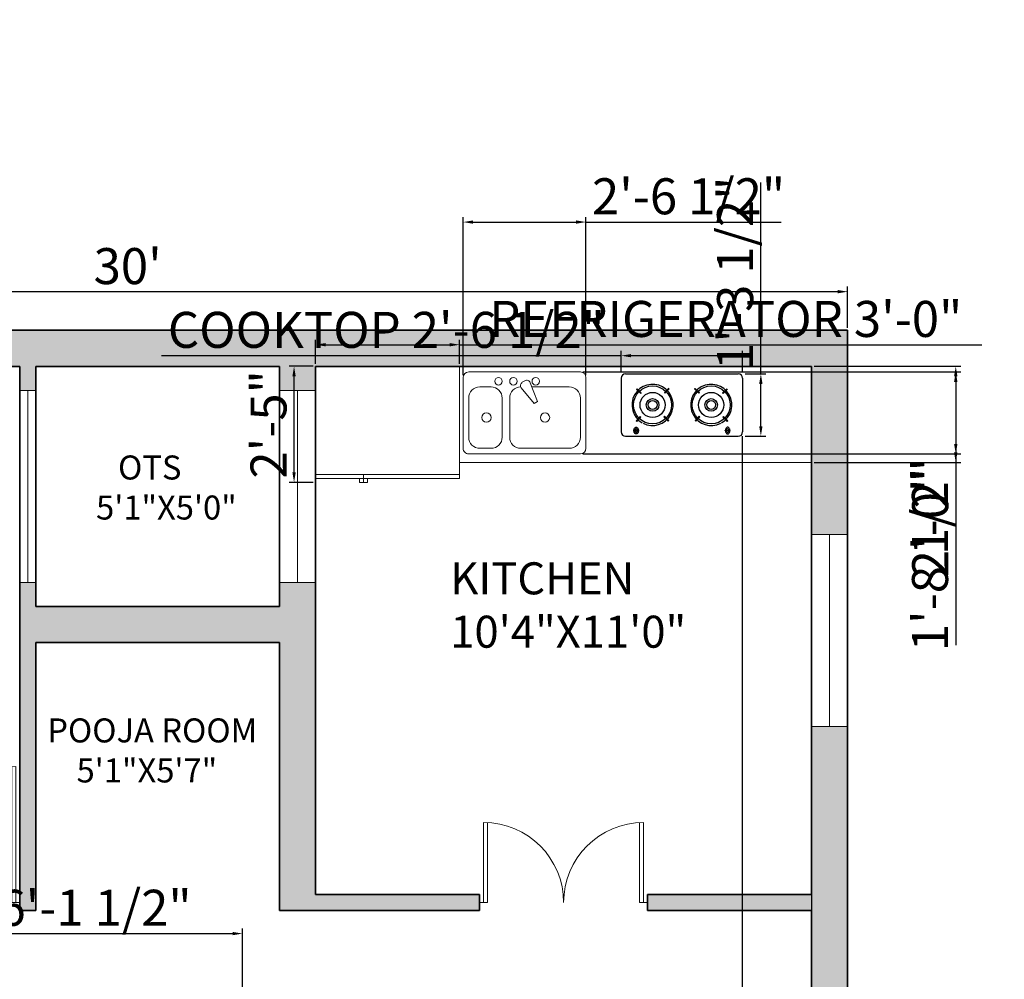
# Model space of a CAD drawing. Units: inches. Extents: x 3592 to 4861, y 1650 to 2243.
# Tile 25 of 30: x 4191 to 4438, y 2003 to 2243. Entities that reach past the tile are written whole.
import ezdxf

# ---------------------------------------------------------------- set-up
doc = ezdxf.new("R2010")
doc.units = ezdxf.units.IN
for name, color, linetype, lineweight in [('A-ANNO-DIMS', 2, 'Continuous', 13), ('A-AREA-IDEN', 7, 'Continuous', 18), ('A-DOOR', 3, 'Continuous', 20), ('A-FLOR-CASE', 7, 'Continuous', 18), ('A-GLAZ', 4, 'Continuous', 18), ('A-WALL', 7, 'Continuous', 35), ('THIET-BI', 21, 'Continuous', 18), ('Сантехника', 9, 'Continuous', 18)]:
    doc.layers.add(name, color=color, linetype=linetype, lineweight=lineweight)
doc.layers.add('A-WALL-PATT', color=252, linetype='Continuous', lineweight=13, true_color=0x939598)
doc.layers.add('NOI THAT', color=42, linetype='Continuous')
doc.styles.add('ATT', font='romans.shx')
doc.styles.get("Standard").update_dxf_attribs({"font": 'arial.ttf'})
doc.dimstyles.new('ISO-25', dxfattribs={"dimtxt": 9, "dimasz": 2.5, "dimexe": 1.25, "dimexo": 0.625, "dimtad": 1, "dimlunit": 3, "dimtxsty": 'Standard', "dimcen": 2.5, "dimadec": 0, "dimazin": 0, "dimtfac": 1, "dimtmove": 0, "dimatfit": 3, "dimfxl": 1, "dimarcsym": 0})

# ---------------------------------------------------------------- blocks, each defined once
blk = doc.blocks.new('1')
for p, q in [((3628.27, 1890.86), (3628.27, 1924.86)), ((3629.27, 1890.86), (3629.27, 1924.86)), ((3627.27, 1890.86), (3629.27, 1890.86)), ((3662.27, 1890.86), (3663.27, 1890.86))]:
    blk.add_line(p, q)
blk.add_arc((3628.27, 1890.86), 34, 0, 90)
blk = doc.blocks.new('MD')
for p, q in [((3665.34, 1831.69), (3665.34, 1851.69)), ((3666.34, 1831.69), (3666.34, 1851.69)), ((3704.34, 1831.69), (3704.34, 1851.69)), ((3705.34, 1831.69), (3705.34, 1851.69)), ((3664.34, 1831.69), (3666.34, 1831.69)), ((3706.34, 1831.69), (3704.34, 1831.69))]:
    blk.add_line(p, q)
for centre, start, end in [((3665.34, 1831.69), 0, 90), ((3705.34, 1831.69), 90, 180)]:
    blk.add_arc(centre, 20, start, end)
blk = doc.blocks.new('*D7')
at = {"layer": 'A-ANNO-DIMS', "color": 0, "lineweight": -2, "transparency": 16777216}
for p, q in [((4038.37, 2165.84), (4038.37, 2176.13)), ((4040.87, 2174.88), (4395.87, 2174.88)), ((4398.37, 2165.84), (4398.37, 2176.13))]:
    blk.add_line(p, q, dxfattribs=at)
at = {"layer": 'A-ANNO-DIMS', "color": 0, "transparency": 16777216}
for points in [[(4040.87, 2175.3), (4040.87, 2174.46), (4038.37, 2174.88)], [(4395.87, 2175.3), (4395.87, 2174.46), (4398.37, 2174.88)]]:
    blk.add_solid(points, dxfattribs=at)
at = {"layer": 'Defpoints', "color": 0, "transparency": 16777216}
for p in [(4398.37, 2174.88), (4038.37, 2165.22), (4398.37, 2165.22)]:
    blk.add_point(p, dxfattribs=at)
at = {"layer": 'A-ANNO-DIMS', "color": 0, "transparency": 16777216, "insert": (4218.37, 2180.1), "char_height": 9, "attachment_point": 5}
blk.add_mtext("30'", dxfattribs=at)
blk = doc.blocks.new('15PSNK11')
at = {"color": 0, "linetype": 'ByBlock'}
for p, q in [((1.5, 16.5), (20.5, 16.5)), ((0, -15), (0, 15)), ((17.5, 15), (7, 15)), ((22, 15), (22, -15)), ((4, 12), (4, 1.954648)), ((20.5, -1), (20.5, 12)), ((2.880753, 1.53534), (7.946152, 3.433013)), ((7.946152, 3.433013), (8.446152, 2.566987)), ((2.365551, 0.098898), (2.768424, -0.598898)), ((8.446152, 2.566987), (4.27002, -0.870941)), ((7, -4), (17.5, -4)), ((17.5, -6), (7, -6)), ((4, -9), (4, -12)), ((20.5, -12), (20.5, -9)), ((7, -15), (17.5, -15)), ((20.5, -16.5), (1.5, -16.5))]:
    blk.add_line(p, q, dxfattribs=at)
for centre, radius in [((12.25, 5.5), 1.25), ((2.5, 3), 1), ((2.5, -3), 1), ((2.5, -7), 1), ((12.25, -10.25), 1.25)]:
    blk.add_circle(centre, radius, dxfattribs=at)
for centre, radius, start, end in [((1.5, 15), 1.5, 90, 180), ((20.5, 15), 1.5, 0, 90), ((7, 12), 3, 90, 180), ((17.5, 12), 3, 0, 90), ((3.231576, 0.598898), 1, 110.537678, 210), ((3.634449, -0.098898), 1, 210, 309.462322), ((7, -1), 3, 180, 270), ((17.5, -1), 3, 270, 0), ((7, -9), 3, 90, 180), ((17.5, -9), 3, 0, 90), ((7, -12), 3, 180, 270), ((17.5, -12), 3, 270, 0), ((1.5, -15), 1.5, 180, 270), ((20.5, -15), 1.5, 270, 0)]:
    blk.add_arc(centre, radius, start, end, dxfattribs=at)
at = {"color": 0, "linetype": 'ByBlock', "style": 'ATT'}
for tag, p, flags in [('ITEM', (0, -26), 3), ('ROOM_NUMBER', (0, -35), 1)]:
    blk.add_attdef(tag, p, '', height=6, dxfattribs=dict(at, flags=flags))
blk = doc.blocks.new('A$C2C6C0730')
at = {"layer": 'NOI THAT'}
for p, q in [((670, 1403), (50, 1403)), ((0, 1353), (0, 50)), ((720, 1353), (720, 50)), ((670, 0), (50, 0))]:
    blk.add_line(p, q, dxfattribs=at)
for points in [[(66, 1257, -0.070182), (81, 1254, -0.081942), (93, 1249, -0.106897), (102, 1239, -0.135195), (105, 1230, -0.135195), (102, 1220, -0.106897), (93, 1210, -0.081942), (81, 1205, -0.070182), (66, 1203, -0.070182), (50, 1205, -0.081942), (38, 1210, -0.106897), (30, 1220, -0.135195), (27, 1230, -0.135195), (30, 1239, -0.106897), (38, 1249, -0.081942), (50, 1254, -0.070182)], [(66, 146, 0.070182), (81, 148, 0.081942), (93, 154, 0.106897), (102, 163, 0.135195), (105, 173, 0.135195), (102, 183, 0.106897), (93, 192, 0.081942), (81, 198, 0.070182), (66, 200, 0.070182), (50, 198, 0.081942), (38, 192, 0.106897), (30, 183, 0.135195), (27, 173, 0.135195), (30, 163, 0.106897), (38, 154, 0.081942), (50, 148, 0.070182)]]:
    blk.add_lwpolyline(points, format="xyb", close=True, dxfattribs=at)
for points in [[(68, 1203), (68, 1257), (62, 1257), (62, 1203)], [(220, 1175), (171, 1223), (179, 1230), (227, 1182)], [(541, 1226), (493, 1177), (500, 1170), (548, 1219)], [(176, 861), (224, 909), (232, 902), (183, 853)], [(497, 897), (546, 849), (553, 856), (505, 904)], [(176, 542), (224, 494), (232, 501), (183, 550)], [(497, 506), (546, 554), (553, 547), (505, 498)], [(220, 228), (171, 180), (179, 172), (227, 221)], [(541, 177), (493, 225), (500, 233), (548, 184)], [(68, 200), (68, 146), (62, 146), (62, 200)]]:
    blk.add_lwpolyline(points, close=True, dxfattribs=at)
for centre, radius in [((362, 1040), 219), ((362, 1040), 145), ((362, 1040), 72.6), ((362, 1040), 51.5), ((362, 363), 219), ((362, 363), 145), ((362, 363), 72.6), ((362, 363), 51.5)]:
    blk.add_circle(centre, radius, dxfattribs=at)
for centre, radius, start, end in [((50, 1353), 50, 90, 180), ((670, 1353), 50, 0, 90), ((362, 1040), 238, 152.4796, 149.9329), ((65, 1230), 19.4, 99.7177, 260.2823), ((65, 1230), 19.4, 279.9102, 80.0898), ((362, 363), 238, 210.0671, 207.5204), ((65, 173), 19.4, 99.7177, 260.2823), ((65, 173), 19.4, 279.9102, 80.0898), ((50, 50), 50, 180, 270), ((670, 50), 50, 270, 0)]:
    blk.add_arc(centre, radius, start, end, dxfattribs=at)
blk = doc.blocks.new('Refrigerator-2 door - 36 in top')
for p, q in [((0, -26.999999), (36, -26.999999)), ((12, -26.999999), (12, -28.999999)), ((11, -27.999999), (11, -28.999999)), ((11, -28.999999), (13, -28.999999)), ((13, -28.999999), (13, -27.999999))]:
    blk.add_line(p, q)
blk.add_lwpolyline([(0, -27.999999), (0, 0), (36, 0), (36, -27.999999)], close=True)
blk = doc.blocks.new('*D155')
at = {"layer": 'A-ANNO-DIMS', "color": 0, "lineweight": -2, "transparency": 16777216}
for p, q in [((4183.77, 2156.22), (4183.77, 2242.84)), ((4169.25, 2156.22), (4185.02, 2156.22)), ((4183.77, 2075.11), (4183.77, 2153.72)), ((4169.25, 2072.61), (4185.02, 2072.61))]:
    blk.add_line(p, q, dxfattribs=at)
at = {"layer": 'A-ANNO-DIMS', "color": 0, "transparency": 16777216}
for points in [[(4183.36, 2153.72), (4184.19, 2153.72), (4183.77, 2156.22)], [(4183.36, 2075.11), (4184.19, 2075.11), (4183.77, 2072.61)]]:
    blk.add_solid(points, dxfattribs=at)
at = {"layer": 'Defpoints', "color": 0, "transparency": 16777216}
for p in [(4168.62, 2156.22), (4183.77, 2156.22), (4168.62, 2072.61)]:
    blk.add_point(p, dxfattribs=at)
at = {"layer": 'A-ANNO-DIMS', "color": 0, "transparency": 16777216, "insert": (4178.5, 2200.78), "char_height": 9, "attachment_point": 5, "rotation": 90}
blk.add_mtext('6\'-11 1/2" TYP.', dxfattribs=at)
blk = doc.blocks.new('*D160')
at = {"layer": 'A-ANNO-DIMS', "color": 0, "lineweight": -2, "transparency": 16777216}
for p, q in [((4341.76, 2154.95), (4341.76, 2160.13)), ((4372.13, 2154.95), (4372.13, 2160.13)), ((4341.76, 2158.88), (4226.85, 2158.88)), ((4369.63, 2158.88), (4344.26, 2158.88))]:
    blk.add_line(p, q, dxfattribs=at)
at = {"layer": 'A-ANNO-DIMS', "color": 0, "transparency": 16777216}
for points in [[(4344.26, 2159.3), (4344.26, 2158.47), (4341.76, 2158.88)], [(4369.63, 2159.3), (4369.63, 2158.47), (4372.13, 2158.88)]]:
    blk.add_solid(points, dxfattribs=at)
at = {"layer": 'Defpoints', "color": 0, "transparency": 16777216}
for p in [(4341.76, 2158.88), (4341.76, 2154.33), (4372.13, 2154.33)]:
    blk.add_point(p, dxfattribs=at)
at = {"layer": 'A-ANNO-DIMS', "color": 0, "transparency": 16777216, "insert": (4283.06, 2164.17), "char_height": 9, "attachment_point": 5}
blk.add_mtext('COOKTOP 2\'-6 1/2"', dxfattribs=at)
blk = doc.blocks.new('*D161')
at = {"layer": 'A-ANNO-DIMS', "color": 0, "lineweight": -2, "transparency": 16777216}
for p, q in [((4376.69, 2154.33), (4376.69, 2202.13)), ((4372.76, 2154.33), (4377.94, 2154.33)), ((4376.69, 2141.24), (4376.69, 2151.83)), ((4372.76, 2138.74), (4377.94, 2138.74))]:
    blk.add_line(p, q, dxfattribs=at)
at = {"layer": 'A-ANNO-DIMS', "color": 0, "transparency": 16777216}
for points in [[(4376.27, 2151.83), (4377.1, 2151.83), (4376.69, 2154.33)], [(4376.27, 2141.24), (4377.1, 2141.24), (4376.69, 2138.74)]]:
    blk.add_solid(points, dxfattribs=at)
at = {"layer": 'Defpoints', "color": 0, "transparency": 16777216}
for p in [(4372.13, 2154.33), (4376.69, 2154.33), (4372.13, 2138.74)]:
    blk.add_point(p, dxfattribs=at)
at = {"layer": 'A-ANNO-DIMS', "color": 0, "transparency": 16777216, "insert": (4371.41, 2179.48), "char_height": 9, "attachment_point": 5, "rotation": 90}
blk.add_mtext('1\'-3 1/2"', dxfattribs=at)
blk = doc.blocks.new('*D162')
at = {"layer": 'A-ANNO-DIMS', "color": 0, "lineweight": -2, "transparency": 16777216}
for p, q in [((4265.37, 2156.84), (4265.37, 2162.87)), ((4267.87, 2161.62), (4298.87, 2161.62)), ((4301.37, 2156.84), (4301.37, 2162.87)), ((4301.37, 2161.62), (4431.96, 2161.62))]:
    blk.add_line(p, q, dxfattribs=at)
at = {"layer": 'A-ANNO-DIMS', "color": 0, "transparency": 16777216}
for points in [[(4267.87, 2162.04), (4267.87, 2161.2), (4265.37, 2161.62)], [(4298.87, 2162.04), (4298.87, 2161.2), (4301.37, 2161.62)]]:
    blk.add_solid(points, dxfattribs=at)
at = {"layer": 'Defpoints', "color": 0, "transparency": 16777216}
for p in [(4301.37, 2161.62), (4265.37, 2156.22), (4301.37, 2156.22)]:
    blk.add_point(p, dxfattribs=at)
at = {"layer": 'A-ANNO-DIMS', "color": 0, "transparency": 16777216, "insert": (4367.92, 2166.9), "char_height": 9, "attachment_point": 5}
blk.add_mtext('REFRIGERATOR 3\'-0"', dxfattribs=at)
blk = doc.blocks.new('*D163')
at = {"layer": 'A-ANNO-DIMS', "color": 0, "lineweight": -2, "transparency": 16777216}
for p, q in [((4264.74, 2156.22), (4258.72, 2156.22)), ((4259.97, 2129.72), (4259.97, 2153.72)), ((4264.74, 2127.22), (4258.72, 2127.22))]:
    blk.add_line(p, q, dxfattribs=at)
at = {"layer": 'A-ANNO-DIMS', "color": 0, "transparency": 16777216}
for points in [[(4259.55, 2153.72), (4260.39, 2153.72), (4259.97, 2156.22)], [(4259.55, 2129.72), (4260.39, 2129.72), (4259.97, 2127.22)]]:
    blk.add_solid(points, dxfattribs=at)
at = {"layer": 'Defpoints', "color": 0, "transparency": 16777216}
for p in [(4259.97, 2156.22), (4265.37, 2156.22), (4265.37, 2127.22)]:
    blk.add_point(p, dxfattribs=at)
at = {"layer": 'A-ANNO-DIMS', "color": 0, "transparency": 16777216, "insert": (4254.75, 2141.72), "char_height": 9, "attachment_point": 5, "rotation": 90}
blk.add_mtext('2\'-5"', dxfattribs=at)
blk = doc.blocks.new('*D165')
at = {"layer": 'A-ANNO-DIMS', "color": 0, "lineweight": -2, "transparency": 16777216}
for p, q in [((4173.35, 1996.55), (4173.35, 2015.72)), ((4175.85, 2014.47), (4244.58, 2014.47)), ((4247.08, 1996.55), (4247.08, 2015.72))]:
    blk.add_line(p, q, dxfattribs=at)
at = {"layer": 'A-ANNO-DIMS', "color": 0, "transparency": 16777216}
for points in [[(4175.85, 2014.88), (4175.85, 2014.05), (4173.35, 2014.47)], [(4244.58, 2014.88), (4244.58, 2014.05), (4247.08, 2014.47)]]:
    blk.add_solid(points, dxfattribs=at)
at = {"layer": 'Defpoints', "color": 0, "transparency": 16777216}
for p in [(4247.08, 2014.47), (4173.35, 1995.93), (4247.08, 1995.93)]:
    blk.add_point(p, dxfattribs=at)
at = {"layer": 'A-ANNO-DIMS', "color": 0, "transparency": 16777216, "insert": (4210.21, 2019.75), "char_height": 9, "attachment_point": 5}
blk.add_mtext('6\'-1 1/2"', dxfattribs=at)
blk = doc.blocks.new('*D170')
at = {"layer": 'A-ANNO-DIMS', "color": 0, "lineweight": -2, "transparency": 16777216}
for p, q in [((4302.25, 2154.04), (4302.25, 2193.52)), ((4304.75, 2192.27), (4330.46, 2192.27)), ((4332.96, 2154.04), (4332.96, 2193.52)), ((4332.96, 2192.27), (4381.76, 2192.27))]:
    blk.add_line(p, q, dxfattribs=at)
at = {"layer": 'A-ANNO-DIMS', "color": 0, "transparency": 16777216}
for points in [[(4304.75, 2192.69), (4304.75, 2191.85), (4302.25, 2192.27)], [(4330.46, 2192.69), (4330.46, 2191.85), (4332.96, 2192.27)]]:
    blk.add_solid(points, dxfattribs=at)
at = {"layer": 'Defpoints', "color": 0, "transparency": 16777216}
for p in [(4332.96, 2192.27), (4302.25, 2153.42), (4332.96, 2153.42)]:
    blk.add_point(p, dxfattribs=at)
at = {"layer": 'A-ANNO-DIMS', "color": 0, "transparency": 16777216, "insert": (4358.61, 2197.55), "char_height": 9, "attachment_point": 5}
blk.add_mtext('2\'-6 1/2"', dxfattribs=at)
blk = doc.blocks.new('*D171')
at = {"layer": 'A-ANNO-DIMS', "color": 0, "lineweight": -2, "transparency": 16777216}
for p, q in [((4332.19, 2154.81), (4426.67, 2154.81)), ((4425.42, 2152.31), (4425.42, 2136.83)), ((4332.19, 2134.33), (4426.67, 2134.33)), ((4425.42, 2134.33), (4425.42, 2086.54))]:
    blk.add_line(p, q, dxfattribs=at)
at = {"layer": 'A-ANNO-DIMS', "color": 0, "transparency": 16777216}
for points in [[(4425, 2152.31), (4425.84, 2152.31), (4425.42, 2154.81)], [(4425, 2136.83), (4425.84, 2136.83), (4425.42, 2134.33)]]:
    blk.add_solid(points, dxfattribs=at)
at = {"layer": 'Defpoints', "color": 0, "transparency": 16777216}
for p in [(4331.57, 2154.81), (4331.57, 2134.33), (4425.42, 2134.33)]:
    blk.add_point(p, dxfattribs=at)
at = {"layer": 'A-ANNO-DIMS', "color": 0, "transparency": 16777216, "insert": (4420.14, 2109.18), "char_height": 9, "attachment_point": 5, "rotation": 90}
blk.add_mtext('1\'-8 1/2"', dxfattribs=at)
blk = doc.blocks.new('*D172')
at = {"layer": 'A-ANNO-DIMS', "color": 0, "lineweight": -2, "transparency": 16777216}
for p, q in [((4389.99, 2156.22), (4426.67, 2156.22)), ((4425.42, 2153.72), (4425.42, 2134.72)), ((4389.99, 2132.22), (4426.67, 2132.22)), ((4425.42, 2132.22), (4425.42, 2104.39))]:
    blk.add_line(p, q, dxfattribs=at)
at = {"layer": 'A-ANNO-DIMS', "color": 0, "transparency": 16777216}
for points in [[(4425, 2153.72), (4425.84, 2153.72), (4425.42, 2156.22)], [(4425, 2134.72), (4425.84, 2134.72), (4425.42, 2132.22)]]:
    blk.add_solid(points, dxfattribs=at)
at = {"layer": 'Defpoints', "color": 0, "transparency": 16777216}
for p in [(4389.37, 2156.22), (4389.37, 2132.22), (4425.42, 2132.22)]:
    blk.add_point(p, dxfattribs=at)
at = {"layer": 'A-ANNO-DIMS', "color": 0, "transparency": 16777216, "insert": (4420.2, 2117.06), "char_height": 9, "attachment_point": 5, "rotation": 90}
blk.add_mtext('2\'-0"', dxfattribs=at)
blk = doc.blocks.new('*D173')
at = {"layer": 'A-ANNO-DIMS', "color": 0, "lineweight": -2, "transparency": 16777216}
for p, q in [((4372.05, 2138.77), (4372.05, 1656.92)), ((4389.37, 2131.59), (4389.37, 1656.92)), ((4374.55, 1658.17), (4386.87, 1658.17)), ((4389.37, 1658.17), (4437.17, 1658.17))]:
    blk.add_line(p, q, dxfattribs=at)
at = {"layer": 'A-ANNO-DIMS', "color": 0, "transparency": 16777216}
for points in [[(4374.55, 1658.59), (4374.55, 1657.75), (4372.05, 1658.17)], [(4386.87, 1658.59), (4386.87, 1657.75), (4389.37, 1658.17)]]:
    blk.add_solid(points, dxfattribs=at)
at = {"layer": 'Defpoints', "color": 0, "transparency": 16777216}
for p in [(4372.05, 2139.4), (4389.37, 2132.22), (4389.37, 1658.17)]:
    blk.add_point(p, dxfattribs=at)
at = {"layer": 'A-ANNO-DIMS', "color": 0, "transparency": 16777216, "insert": (4414.52, 1663.45), "char_height": 9, "attachment_point": 5}
blk.add_mtext('1\'-5 1/2"', dxfattribs=at)

msp = doc.modelspace()

# ---------------------------------------------------------------- hatches: boundary and pattern name
at = {"layer": 'A-WALL-PATT'}
h = msp.add_hatch(color=256, dxfattribs=at)
h.dxf.hatch_style = 1
h.paths.add_polyline_path([(4398.37, 2165.219), (4038.37, 2165.219), (4038.37, 1993.219), (4047.37, 1993.219), (4047.37, 2156.219), (4191.37, 2156.219), (4191.37, 2150.219), (4195.37, 2150.219), (4195.37, 2156.219), (4256.37, 2156.219), (4256.37, 2150.219), (4265.37, 2150.219), (4265.37, 2156.219), (4389.37, 2156.219), (4389.37, 2114.219), (4398.37, 2114.219)])
h.paths.add_polyline_path([(4265.37, 2102.219), (4256.37, 2102.219), (4256.37, 2096.219), (4195.37, 2096.219), (4195.37, 2102.219), (4191.37, 2102.219), (4191.37, 2020.219), (4195.37, 2020.219), (4195.37, 2087.219), (4256.37, 2087.219), (4256.37, 2020.219), (4306.37, 2020.219), (4306.37, 2024.219), (4265.37, 2024.219)], flags=17)
h.paths.add_polyline_path([(4398.37, 2066.219), (4389.37, 2066.219), (4389.37, 2024.219), (4348.37, 2024.219), (4348.37, 2020.219), (4389.37, 2020.219), (4389.37, 1989.719), (4398.37, 1989.719)])
h.paths.add_polyline_path([(4398.37, 1941.719), (4389.37, 1941.719), (4389.37, 1911.219), (4301.37, 1911.219), (4301.37, 1907.219), (4389.37, 1907.219), (4389.37, 1865.219), (4398.37, 1865.219)])
h.paths.add_polyline_path([(4398.37, 1817.219), (4389.37, 1817.219), (4389.37, 1775.219), (4265.37, 1775.219), (4265.37, 1911.219), (4256.37, 1911.219), (4256.37, 1817.219), (4220.87, 1817.219), (4220.87, 1808.219), (4256.37, 1808.219), (4256.37, 1766.219), (4389.37, 1766.219), (4389.37, 1694.219), (4256.37, 1694.219), (4256.37, 1685.219), (4398.37, 1685.219)])
h.paths.add_polyline_path([(4178.87, 1817.219), (4077.37, 1817.219), (4077.37, 1808.219), (4178.87, 1808.219)])
h.paths.add_polyline_path([(4111.37, 2020.219), (4155.37, 2020.219), (4155.37, 2024.219), (4077.37, 2024.219), (4077.37, 2020.219), (4107.37, 2020.219), (4107.37, 1942.219), (4047.37, 1942.219), (4047.37, 1969.219), (4038.37, 1969.219), (4038.37, 1911.219), (4047.37, 1911.219), (4047.37, 1938.219), (4107.37, 1938.219), (4107.37, 1860.219), (4077.37, 1860.219), (4077.37, 1856.219), (4111.37, 1856.219)])
h.paths.add_polyline_path([(4047.37, 1887.219), (4038.37, 1887.219), (4038.37, 1685.219), (4152.37, 1685.219), (4152.37, 1715.219), (4143.37, 1715.219), (4143.37, 1694.219), (4047.37, 1694.219)])
h.paths.add_polyline_path([(4152.37, 1772.219), (4143.37, 1772.219), (4143.37, 1751.219), (4152.37, 1751.219)], flags=17)

# ---------------------------------------------------------------- linework, layer by layer
at = {"layer": 'A-FLOR-CASE'}
msp.add_line((4301.37, 2132.219), (4389.37, 2132.219), dxfattribs=at)
at = {"layer": 'A-GLAZ'}
for p, q in [((4195.37, 2150.219), (4191.37, 2150.219)), ((4193.37, 2150.219), (4193.37, 2102.219)), ((4265.37, 2150.219), (4256.37, 2150.219)), ((4260.87, 2150.219), (4260.87, 2102.219)), ((4389.37, 2114.219), (4398.37, 2114.219)), ((4393.87, 2114.219), (4393.87, 2066.219)), ((4195.37, 2102.219), (4191.37, 2102.219)), ((4265.37, 2102.219), (4256.37, 2102.219)), ((4389.37, 2066.219), (4398.37, 2066.219))]:
    msp.add_line(p, q, dxfattribs=at)
at = {"layer": 'A-WALL'}
for p, q in [((4038.37, 2165.219), (4398.37, 2165.219)), ((4398.37, 2165.219), (4398.37, 1685.219)), ((4047.37, 2156.219), (4191.37, 2156.219)), ((4191.37, 2020.219), (4191.37, 2156.219)), ((4195.37, 2156.219), (4256.37, 2156.219)), ((4195.37, 2096.219), (4195.37, 2156.219)), ((4256.37, 2156.219), (4256.37, 2096.219)), ((4265.37, 2156.219), (4389.37, 2156.219)), ((4265.37, 2156.219), (4265.37, 2024.219)), ((4389.37, 2156.219), (4389.37, 2024.219)), ((4195.37, 2096.219), (4256.37, 2096.219)), ((4195.37, 2087.219), (4256.37, 2087.219)), ((4195.37, 2020.219), (4195.37, 2087.219)), ((4256.37, 2087.219), (4256.37, 2020.219)), ((4265.37, 2024.219), (4306.37, 2024.219)), ((4306.37, 2024.219), (4306.37, 2020.219)), ((4348.37, 2024.219), (4389.37, 2024.219)), ((4348.37, 2024.219), (4348.37, 2020.219)), ((4191.37, 2020.219), (4195.37, 2020.219)), ((4256.37, 2020.219), (4306.37, 2020.219)), ((4348.37, 2020.219), (4389.37, 2020.219)), ((4389.37, 2020.219), (4389.37, 1911.219))]:
    msp.add_line(p, q, dxfattribs=at)

# ---------------------------------------------------------------- block references
at = {"layer": 'A-DOOR', "xscale": -1}
msp.add_blockref('1', (7818.637, 131.354), dxfattribs=at)
at = {"layer": 'A-DOOR'}
msp.add_blockref('MD', (642.034, 190.53), dxfattribs=at)
at = {"layer": 'THIET-BI'}
msp.add_blockref('Refrigerator-2 door - 36 in top', (4265.37, 2156.219), dxfattribs=at)
at = {"layer": 'THIET-BI', "xscale": 0.021652603804716, "yscale": 0.021652603804716, "zscale": 0.021652603804716, "rotation": 90}
msp.add_blockref('A$C2C6C0730', (4372.131, 2138.738), dxfattribs=at)
at = {"layer": 'Сантехника', "xscale": 0.930794468634925, "yscale": 0.930794468634925, "zscale": 0.930794468634925, "rotation": 270}
msp.add_blockref('15PSNK11', (4317.605, 2154.812), dxfattribs=at)

# ---------------------------------------------------------------- texts
at = {"layer": 'A-AREA-IDEN', "attachment_point": 1}
for s, insert, char_height in [('   OTS\\P5\'1"X5\'0"', (4210.463, 2133.938), 6), ('KITCHEN\\P10\'4"X11\'0"', (4299.018, 2107.241), 8), ('POOJA ROOM\\P    5\'1"X5\'7"', (4198.249, 2068.232), 6)]:
    msp.add_mtext_dynamic_manual_height_columns(s, width=121.44943, gutter_width=12.5, heights=[0], dxfattribs=dict(at, insert=insert, char_height=char_height))

# ---------------------------------------------------------------- dimensions: what is measured, and where the dimension line sits
at = {"layer": 'A-ANNO-DIMS'}
for base, p1, p2, angle, text, picture, middle in [((4183.774, 2156.219), (4168.621, 2072.607), (4168.621, 2156.219), 90, '<> TYP.', '*D155', (4178.495, 2200.78)), ((4341.758, 2158.884), (4372.131, 2154.328), (4341.758, 2154.328), 180, 'COOKTOP <>', '*D160', (4283.055, 2164.165))]:
    dim = msp.add_linear_dim(base=base, p1=p1, p2=p2, angle=angle, text=text, dimstyle='ISO-25', override={"dimdec": 1, "dimlfac": 1, "dimrnd": 0, "dimzin": 1, "dimdsep": 46, "dimlunit": 4, "dimfrac": 2}, dxfattribs=at)
    dim.commit()
    dim.dimension.update_dxf_attribs({"geometry": picture, "text_midpoint": middle})
for base, p1, p2, override, picture, middle in [((4332.963, 2192.269), (4302.247, 2153.415), (4332.963, 2153.415), {"dimdec": 1, "dimlfac": 1, "dimrnd": 0, "dimzin": 1, "dimdsep": 46, "dimlunit": 4, "dimfrac": 2}, '*D170', (4358.613, 2197.547)), ((4398.37, 2174.88), (4038.37, 2165.219), (4398.37, 2165.219), {"dimclrd": 0, "dimclre": 0, "dimclrt": 0}, '*D7', (4218.37, 2180.103)), ((4389.37, 1658.169), (4372.046, 2139.399), (4389.37, 2132.219), {"dimdec": 1, "dimlfac": 1, "dimrnd": 0, "dimzin": 1, "dimdsep": 46, "dimlunit": 4, "dimfrac": 2}, '*D173', (4414.519, 1663.447)), ((4247.079, 2014.467), (4173.347, 1995.926), (4247.079, 1995.926), {"dimdec": 1, "dimlfac": 1, "dimrnd": 0, "dimzin": 1, "dimdsep": 46, "dimlunit": 4, "dimfrac": 2}, '*D165', (4210.213, 2019.746))]:
    dim = msp.add_linear_dim(base=base, p1=p1, p2=p2, dimstyle='ISO-25', override=override, dxfattribs=at)
    dim.commit()
    dim.dimension.update_dxf_attribs({"geometry": picture, "text_midpoint": middle})
for base, p1, p2, picture, middle in [((4376.687, 2154.328), (4372.131, 2138.738), (4372.131, 2154.328), '*D161', (4371.405, 2179.477)), ((4259.97, 2156.219), (4265.37, 2127.219), (4265.37, 2156.219), '*D163', (4254.75, 2141.719)), ((4425.42, 2134.334), (4331.567, 2154.812), (4331.567, 2134.334), '*D171', (4420.141, 2109.185)), ((4425.42, 2132.219), (4389.37, 2156.219), (4389.37, 2132.219), '*D172', (4420.2, 2117.055))]:
    dim = msp.add_linear_dim(base=base, p1=p1, p2=p2, angle=90, dimstyle='ISO-25', override={"dimdec": 1, "dimlfac": 1, "dimrnd": 0, "dimzin": 1, "dimdsep": 46, "dimlunit": 4, "dimfrac": 2}, dxfattribs=at)
    dim.commit()
    dim.dimension.update_dxf_attribs({"geometry": picture, "text_midpoint": middle})
dim = msp.add_linear_dim(base=(4301.37, 2161.619), p1=(4265.37, 2156.219), p2=(4301.37, 2156.219), text='REFRIGERATOR <>', dimstyle='ISO-25', override={"dimdec": 1, "dimlfac": 1, "dimrnd": 0, "dimzin": 1, "dimdsep": 46, "dimlunit": 4, "dimfrac": 2}, dxfattribs=at)
dim.commit()
dim.dimension.update_dxf_attribs({"geometry": '*D162', "text_midpoint": (4367.915, 2166.904)})

doc.saveas('drawing.dxf')
